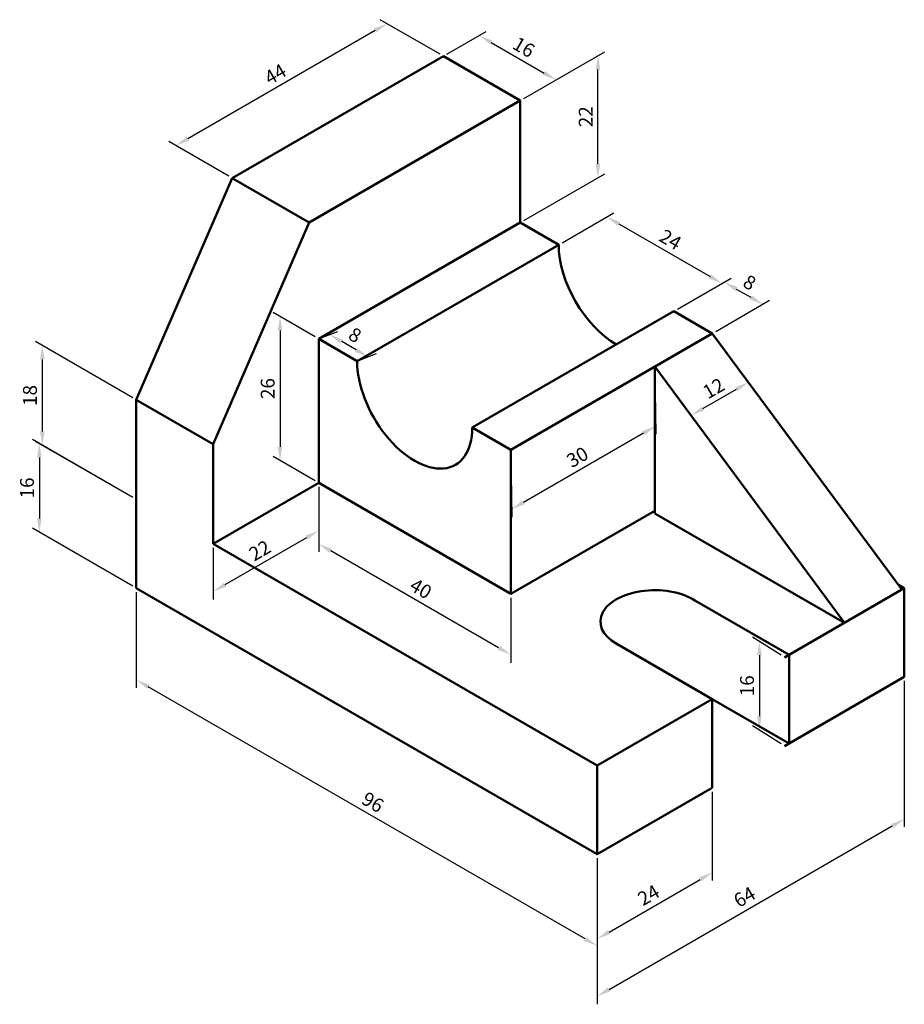
# Model space of a CAD drawing. Units: millimetres. Extents: x 27507 to 27667, y 10668 to 10845.
import ezdxf

# ---------------------------------------------------------------- set-up
doc = ezdxf.new("R2010")
doc.units = ezdxf.units.MM
doc.layers.add('M-DIMS', color=2, linetype='Continuous', lineweight=25)
doc.layers.add('M-OUTL', color=7, linetype='Continuous', lineweight=50)
doc.styles.get("Standard").update_dxf_attribs({"font": 'arial.ttf'})
doc.dimstyles.new('ISO-25', dxfattribs={"dimtxt": 2.5, "dimasz": 2.5, "dimexe": 1.25, "dimexo": 0.625, "dimtad": 1, "dimtxsty": 'Standard', "dimcen": 2.5, "dimadec": 0, "dimazin": 0, "dimtfac": 1, "dimtmove": 0, "dimatfit": 3, "dimfxl": 1, "dimarcsym": 0})

# ---------------------------------------------------------------- blocks, each defined once
blk = doc.blocks.new('*D1')
at = {"layer": 'Defpoints', "color": 0, "transparency": 16777216}
for p in [(27528.09, 10742.67), (27528.09, 10726.14), (27611.23, 10694.67)]:
    blk.add_point(p, dxfattribs=at)
at = {"layer": 'M-DIMS', "color": 0, "lineweight": -2, "transparency": 16777216}
for p, q in [((27528.09, 10741.95), (27528.09, 10724.69)), ((27609.06, 10679.39), (27530.26, 10724.89)), ((27611.23, 10693.95), (27611.23, 10676.69))]:
    blk.add_line(p, q, dxfattribs=at)
at = {"layer": 'M-DIMS', "color": 0, "transparency": 16777216}
for points in [[(27530.46, 10725.25), (27530.05, 10724.53), (27528.09, 10726.14)], [(27609.27, 10679.75), (27608.86, 10679.03), (27611.23, 10678.14)]]:
    blk.add_solid(points, dxfattribs=at)
at = {"layer": 'M-DIMS', "color": 0, "transparency": 16777216, "insert": (27570.61, 10703.78), "char_height": 2.5, "attachment_point": 5, "rotation": 330}
blk.add_mtext('96', dxfattribs=at)
blk = doc.blocks.new('*D2')
at = {"layer": 'Defpoints', "color": 0, "transparency": 16777216}
for p in [(27632.01, 10706.67), (27611.23, 10694.67), (27632.01, 10691.38)]:
    blk.add_point(p, dxfattribs=at)
at = {"layer": 'M-DIMS', "color": 0, "lineweight": -2, "transparency": 16777216}
for p, q in [((27632.01, 10705.95), (27632.01, 10689.94)), ((27611.23, 10693.95), (27611.23, 10677.94)), ((27613.39, 10680.63), (27629.85, 10690.13))]:
    blk.add_line(p, q, dxfattribs=at)
at = {"layer": 'M-DIMS', "color": 0, "transparency": 16777216}
for points in [[(27629.64, 10690.49), (27630.06, 10689.77), (27632.01, 10691.38)], [(27613.19, 10680.99), (27613.6, 10680.27), (27611.23, 10679.38)]]:
    blk.add_solid(points, dxfattribs=at)
at = {"layer": 'M-DIMS', "color": 0, "transparency": 16777216, "insert": (27620.68, 10687.01), "char_height": 2.5, "attachment_point": 5, "rotation": 30}
blk.add_mtext('24', dxfattribs=at)
blk = doc.blocks.new('*D3')
at = {"layer": 'Defpoints', "color": 0, "transparency": 16777216}
for p in [(27645.04, 10730.19), (27640.5, 10717.07), (27645.04, 10714.19)]:
    blk.add_point(p, dxfattribs=at)
at = {"layer": 'M-DIMS', "color": 0, "lineweight": -2, "transparency": 16777216}
for p, q in [((27644.41, 10730.58), (27639.25, 10733.86)), ((27640.5, 10730.57), (27640.5, 10719.57)), ((27644.41, 10714.58), (27639.25, 10717.86))]:
    blk.add_line(p, q, dxfattribs=at)
at = {"layer": 'M-DIMS', "color": 0, "transparency": 16777216}
for points in [[(27640.09, 10730.57), (27640.92, 10730.57), (27640.5, 10733.07)], [(27640.09, 10719.57), (27640.92, 10719.57), (27640.5, 10717.07)]]:
    blk.add_solid(points, dxfattribs=at)
at = {"layer": 'M-DIMS', "color": 0, "transparency": 16777216, "insert": (27638.6, 10725.07), "char_height": 2.5, "attachment_point": 5, "rotation": 90}
blk.add_mtext('16', dxfattribs=at)
blk = doc.blocks.new('*D4')
at = {"layer": 'Defpoints', "color": 0, "transparency": 16777216}
for p in [(27666.65, 10726.67), (27666.65, 10701.03), (27611.23, 10694.67)]:
    blk.add_point(p, dxfattribs=at)
at = {"layer": 'M-DIMS', "color": 0, "lineweight": -2, "transparency": 16777216}
for p, q in [((27666.65, 10725.95), (27666.65, 10699.59)), ((27613.39, 10670.28), (27664.49, 10699.78)), ((27611.23, 10693.95), (27611.23, 10667.59))]:
    blk.add_line(p, q, dxfattribs=at)
at = {"layer": 'M-DIMS', "color": 0, "transparency": 16777216}
for points in [[(27664.28, 10700.14), (27664.7, 10699.42), (27666.65, 10701.03)], [(27613.19, 10670.64), (27613.6, 10669.92), (27611.23, 10669.03)]]:
    blk.add_solid(points, dxfattribs=at)
at = {"layer": 'M-DIMS', "color": 0, "transparency": 16777216, "insert": (27637.99, 10686.68), "char_height": 2.5, "attachment_point": 5, "rotation": 30}
blk.add_mtext('64', dxfattribs=at)
blk = doc.blocks.new('*D5')
at = {"layer": 'Defpoints', "color": 0, "transparency": 16777216}
for p in [(27632.01, 10788.67), (27621.62, 10782.67), (27638.55, 10779.84)]:
    blk.add_point(p, dxfattribs=at)
at = {"layer": 'M-DIMS', "color": 0, "lineweight": -2, "transparency": 16777216}
for p, q in [((27632.39, 10788.16), (27639.29, 10778.83)), ((27621.99, 10782.16), (27628.9, 10772.83)), ((27630.32, 10775.09), (27636.38, 10778.59))]:
    blk.add_line(p, q, dxfattribs=at)
at = {"layer": 'M-DIMS', "color": 0, "transparency": 16777216}
for points in [[(27636.17, 10778.95), (27636.59, 10778.23), (27638.55, 10779.84)], [(27630.11, 10775.45), (27630.53, 10774.73), (27628.15, 10773.84)]]:
    blk.add_solid(points, dxfattribs=at)
at = {"layer": 'M-DIMS', "color": 0, "transparency": 16777216, "insert": (27632.41, 10778.47), "char_height": 2.5, "attachment_point": 5, "rotation": 30}
blk.add_mtext('12', dxfattribs=at)
blk = doc.blocks.new('*D6')
at = {"layer": 'Defpoints', "color": 0, "transparency": 16777216}
for p in [(27641.11, 10793.92), (27625.08, 10792.67), (27632.01, 10788.67)]:
    blk.add_point(p, dxfattribs=at)
at = {"layer": 'M-DIMS', "color": 0, "lineweight": -2, "transparency": 16777216}
for p, q in [((27625.71, 10793.03), (27635.43, 10798.64)), ((27636.34, 10796.67), (27638.94, 10795.17)), ((27632.64, 10789.03), (27642.36, 10794.64))]:
    blk.add_line(p, q, dxfattribs=at)
at = {"layer": 'M-DIMS', "color": 0, "transparency": 16777216}
for points in [[(27636.55, 10797.03), (27636.14, 10796.31), (27634.18, 10797.92)], [(27639.15, 10795.53), (27638.73, 10794.81), (27641.11, 10793.92)]]:
    blk.add_solid(points, dxfattribs=at)
at = {"layer": 'M-DIMS', "color": 0, "transparency": 16777216, "insert": (27638.59, 10797.57), "char_height": 2.5, "attachment_point": 5, "rotation": 330}
blk.add_mtext('8', dxfattribs=at)
blk = doc.blocks.new('*D7')
at = {"layer": 'Defpoints', "color": 0, "transparency": 16777216}
for p in [(27604.3, 10804.67), (27633.76, 10797.68), (27625.08, 10792.67)]:
    blk.add_point(p, dxfattribs=at)
at = {"layer": 'M-DIMS', "color": 0, "lineweight": -2, "transparency": 16777216}
for p, q in [((27604.93, 10805.03), (27614.23, 10810.4)), ((27615.14, 10808.43), (27631.6, 10798.93)), ((27625.71, 10793.03), (27635.01, 10798.4))]:
    blk.add_line(p, q, dxfattribs=at)
at = {"layer": 'M-DIMS', "color": 0, "transparency": 16777216}
for points in [[(27615.35, 10808.79), (27614.93, 10808.07), (27612.98, 10809.68)], [(27631.81, 10799.29), (27631.39, 10798.57), (27633.76, 10797.68)]]:
    blk.add_solid(points, dxfattribs=at)
at = {"layer": 'M-DIMS', "color": 0, "transparency": 16777216, "insert": (27624.31, 10805.31), "char_height": 2.5, "attachment_point": 5, "rotation": 330}
blk.add_mtext('24', dxfattribs=at)
blk = doc.blocks.new('*D8')
at = {"layer": 'Defpoints', "color": 0, "transparency": 16777216}
for p in [(27611.38, 10838.76), (27597.37, 10830.67), (27597.37, 10808.67)]:
    blk.add_point(p, dxfattribs=at)
at = {"layer": 'M-DIMS', "color": 0, "lineweight": -2, "transparency": 16777216}
for p, q in [((27598, 10831.03), (27612.63, 10839.48)), ((27611.38, 10819.26), (27611.38, 10836.26)), ((27598, 10809.03), (27612.63, 10817.48))]:
    blk.add_line(p, q, dxfattribs=at)
at = {"layer": 'M-DIMS', "color": 0, "transparency": 16777216}
for points in [[(27610.96, 10836.26), (27611.8, 10836.26), (27611.38, 10838.76)], [(27610.96, 10819.26), (27611.8, 10819.26), (27611.38, 10816.76)]]:
    blk.add_solid(points, dxfattribs=at)
at = {"layer": 'M-DIMS', "color": 0, "transparency": 16777216, "insert": (27609.5, 10827.76), "char_height": 2.5, "attachment_point": 5, "rotation": 90}
blk.add_mtext('22', dxfattribs=at)
blk = doc.blocks.new('*D9')
at = {"layer": 'Defpoints', "color": 0, "transparency": 16777216}
for p in [(27583.52, 10838.67), (27603.83, 10834.4), (27597.37, 10830.67)]:
    blk.add_point(p, dxfattribs=at)
at = {"layer": 'M-DIMS', "color": 0, "lineweight": -2, "transparency": 16777216}
for p, q in [((27584.14, 10839.03), (27591.22, 10843.12)), ((27592.14, 10841.15), (27601.66, 10835.65)), ((27598, 10831.03), (27605.08, 10835.12))]:
    blk.add_line(p, q, dxfattribs=at)
at = {"layer": 'M-DIMS', "color": 0, "transparency": 16777216}
for points in [[(27592.35, 10841.51), (27591.93, 10840.79), (27589.97, 10842.4)], [(27601.87, 10836.01), (27601.46, 10835.29), (27603.83, 10834.4)]]:
    blk.add_solid(points, dxfattribs=at)
at = {"layer": 'M-DIMS', "color": 0, "transparency": 16777216, "insert": (27597.85, 10840.04), "char_height": 2.5, "attachment_point": 5, "rotation": 330}
blk.add_mtext('16', dxfattribs=at)
blk = doc.blocks.new('*D10')
at = {"layer": 'Defpoints', "color": 0, "transparency": 16777216}
for p in [(27583.52, 10838.67), (27535.22, 10822.55), (27545.41, 10816.67)]:
    blk.add_point(p, dxfattribs=at)
at = {"layer": 'M-DIMS', "color": 0, "lineweight": -2, "transparency": 16777216}
for p, q in [((27582.89, 10839.03), (27572.08, 10845.27)), ((27571.16, 10843.3), (27537.39, 10823.8)), ((27544.79, 10817.03), (27533.97, 10823.27))]:
    blk.add_line(p, q, dxfattribs=at)
at = {"layer": 'M-DIMS', "color": 0, "transparency": 16777216}
for points in [[(27570.96, 10843.66), (27571.37, 10842.94), (27573.33, 10844.55)], [(27537.18, 10824.16), (27537.6, 10823.44), (27535.22, 10822.55)]]:
    blk.add_solid(points, dxfattribs=at)
at = {"layer": 'M-DIMS', "color": 0, "transparency": 16777216, "insert": (27553.34, 10835.17), "char_height": 2.5, "attachment_point": 5, "rotation": 30}
blk.add_mtext('44', dxfattribs=at)
blk = doc.blocks.new('*D11')
at = {"layer": 'Defpoints', "color": 0, "transparency": 16777216}
for p in [(27528.09, 10776.67), (27511.13, 10768.46), (27528.09, 10758.67)]:
    blk.add_point(p, dxfattribs=at)
at = {"layer": 'M-DIMS', "color": 0, "lineweight": -2, "transparency": 16777216}
for p, q in [((27527.46, 10777.03), (27509.88, 10787.18)), ((27511.13, 10783.96), (27511.13, 10770.96)), ((27527.46, 10759.03), (27509.88, 10769.18))]:
    blk.add_line(p, q, dxfattribs=at)
at = {"layer": 'M-DIMS', "color": 0, "transparency": 16777216}
for points in [[(27510.72, 10783.96), (27511.55, 10783.96), (27511.13, 10786.46)], [(27510.72, 10770.96), (27511.55, 10770.96), (27511.13, 10768.46)]]:
    blk.add_solid(points, dxfattribs=at)
at = {"layer": 'M-DIMS', "color": 0, "transparency": 16777216, "insert": (27509.23, 10777.46), "char_height": 2.5, "attachment_point": 5, "rotation": 90}
blk.add_mtext('18', dxfattribs=at)
blk = doc.blocks.new('*D12')
at = {"layer": 'Defpoints', "color": 0, "transparency": 16777216}
for p in [(27528.09, 10758.67), (27510.6, 10752.77), (27528.09, 10742.67)]:
    blk.add_point(p, dxfattribs=at)
at = {"layer": 'M-DIMS', "color": 0, "lineweight": -2, "transparency": 16777216}
for p, q in [((27527.46, 10759.03), (27509.35, 10769.49)), ((27510.6, 10766.27), (27510.6, 10755.27)), ((27527.46, 10743.03), (27509.35, 10753.49))]:
    blk.add_line(p, q, dxfattribs=at)
at = {"layer": 'M-DIMS', "color": 0, "transparency": 16777216}
for points in [[(27510.18, 10766.27), (27511.01, 10766.27), (27510.6, 10768.77)], [(27510.18, 10755.27), (27511.01, 10755.27), (27510.6, 10752.77)]]:
    blk.add_solid(points, dxfattribs=at)
at = {"layer": 'M-DIMS', "color": 0, "transparency": 16777216, "insert": (27508.7, 10760.77), "char_height": 2.5, "attachment_point": 5, "rotation": 90}
blk.add_mtext('16', dxfattribs=at)
blk = doc.blocks.new('*D13')
at = {"layer": 'Defpoints', "color": 0, "transparency": 16777216}
for p in [(27561, 10761.67), (27561, 10753.07), (27541.95, 10750.67)]:
    blk.add_point(p, dxfattribs=at)
at = {"layer": 'M-DIMS', "color": 0, "lineweight": -2, "transparency": 16777216}
for p, q in [((27561, 10760.95), (27561, 10751.63)), ((27544.11, 10743.32), (27558.83, 10751.82)), ((27541.95, 10749.95), (27541.95, 10740.63))]:
    blk.add_line(p, q, dxfattribs=at)
at = {"layer": 'M-DIMS', "color": 0, "transparency": 16777216}
for points in [[(27558.63, 10752.18), (27559.04, 10751.46), (27561, 10753.07)], [(27543.9, 10743.68), (27544.32, 10742.96), (27541.95, 10742.07)]]:
    blk.add_solid(points, dxfattribs=at)
at = {"layer": 'M-DIMS', "color": 0, "transparency": 16777216, "insert": (27550.53, 10749.2), "char_height": 2.5, "attachment_point": 5, "rotation": 30}
blk.add_mtext('22', dxfattribs=at)
blk = doc.blocks.new('*D14')
at = {"layer": 'Defpoints', "color": 0, "transparency": 16777216}
for p in [(27561, 10761.67), (27561, 10750.67), (27595.64, 10741.67)]:
    blk.add_point(p, dxfattribs=at)
at = {"layer": 'M-DIMS', "color": 0, "lineweight": -2, "transparency": 16777216}
for p, q in [((27561, 10760.95), (27561, 10749.23)), ((27593.47, 10731.92), (27563.16, 10749.42)), ((27595.64, 10740.95), (27595.64, 10729.23))]:
    blk.add_line(p, q, dxfattribs=at)
at = {"layer": 'M-DIMS', "color": 0, "transparency": 16777216}
for points in [[(27563.37, 10749.78), (27562.96, 10749.06), (27561, 10750.67)], [(27593.68, 10732.28), (27593.27, 10731.56), (27595.64, 10730.67)]]:
    blk.add_solid(points, dxfattribs=at)
at = {"layer": 'M-DIMS', "color": 0, "transparency": 16777216, "insert": (27579.27, 10742.32), "char_height": 2.5, "attachment_point": 5, "rotation": 330}
blk.add_mtext('40', dxfattribs=at)
blk = doc.blocks.new('*D15')
at = {"layer": 'Defpoints', "color": 0, "transparency": 16777216}
for p in [(27561, 10787.67), (27554.02, 10765.7), (27561, 10761.67)]:
    blk.add_point(p, dxfattribs=at)
at = {"layer": 'M-DIMS', "color": 0, "lineweight": -2, "transparency": 16777216}
for p, q in [((27560.37, 10788.03), (27552.77, 10792.42)), ((27554.02, 10789.2), (27554.02, 10768.2)), ((27560.37, 10762.03), (27552.77, 10766.42))]:
    blk.add_line(p, q, dxfattribs=at)
at = {"layer": 'M-DIMS', "color": 0, "transparency": 16777216}
for points in [[(27553.6, 10789.2), (27554.44, 10789.2), (27554.02, 10791.7)], [(27553.6, 10768.2), (27554.44, 10768.2), (27554.02, 10765.7)]]:
    blk.add_solid(points, dxfattribs=at)
at = {"layer": 'M-DIMS', "color": 0, "transparency": 16777216, "insert": (27552.12, 10778.7), "char_height": 2.5, "attachment_point": 5, "rotation": 90}
blk.add_mtext('26', dxfattribs=at)
blk = doc.blocks.new('*D16')
at = {"layer": 'Defpoints', "color": 0, "transparency": 16777216}
for p in [(27561, 10787.67), (27562.98, 10788.43), (27567.93, 10783.67)]:
    blk.add_point(p, dxfattribs=at)
at = {"layer": 'M-DIMS', "color": 0, "lineweight": -2, "transparency": 16777216}
for p, q in [((27561.75, 10787.96), (27564.48, 10789.01)), ((27567.75, 10785.68), (27565.15, 10787.18)), ((27568.68, 10783.96), (27571.41, 10785.01))]:
    blk.add_line(p, q, dxfattribs=at)
at = {"layer": 'M-DIMS', "color": 0, "transparency": 16777216}
for points in [[(27565.36, 10787.54), (27564.94, 10786.82), (27562.98, 10788.43)], [(27567.95, 10786.04), (27567.54, 10785.32), (27569.91, 10784.43)]]:
    blk.add_solid(points, dxfattribs=at)
at = {"layer": 'M-DIMS', "color": 0, "transparency": 16777216, "insert": (27567.4, 10788.08), "char_height": 2.5, "attachment_point": 5, "rotation": 330}
blk.add_mtext('8', dxfattribs=at)
blk = doc.blocks.new('*D17')
at = {"layer": 'Defpoints', "color": 0, "transparency": 16777216}
for p in [(27621.62, 10782.67), (27595.64, 10767.67), (27595.8, 10756.91)]:
    blk.add_point(p, dxfattribs=at)
at = {"layer": 'M-DIMS', "color": 0, "lineweight": -2, "transparency": 16777216}
for p, q in [((27621.63, 10781.95), (27621.8, 10770.48)), ((27619.61, 10770.66), (27597.96, 10758.16)), ((27595.65, 10766.95), (27595.82, 10755.48))]:
    blk.add_line(p, q, dxfattribs=at)
at = {"layer": 'M-DIMS', "color": 0, "transparency": 16777216}
for points in [[(27619.4, 10771.03), (27619.82, 10770.3), (27621.78, 10771.91)], [(27597.75, 10758.53), (27598.17, 10757.8), (27595.8, 10756.91)]]:
    blk.add_solid(points, dxfattribs=at)
at = {"layer": 'M-DIMS', "color": 0, "transparency": 16777216, "insert": (27607.84, 10766.06), "char_height": 2.5, "attachment_point": 5, "rotation": 30}
blk.add_mtext('30', dxfattribs=at)

msp = doc.modelspace()

# ---------------------------------------------------------------- linework, layer by layer
at = {"layer": 'M-OUTL'}
for p, q in [((27545.41, 10816.668), (27583.516, 10838.668)), ((27583.516, 10838.668), (27597.372, 10830.668)), ((27597.372, 10830.668), (27559.267, 10808.668)), ((27597.372, 10830.668), (27597.372, 10808.668)), ((27545.41, 10816.668), (27528.09, 10776.668)), ((27559.267, 10808.668), (27545.41, 10816.668)), ((27559.267, 10808.668), (27541.946, 10768.668)), ((27560.999, 10787.668), (27597.372, 10808.668)), ((27597.372, 10808.668), (27604.3, 10804.668)), ((27604.3, 10804.668), (27597.372, 10808.668)), ((27567.927, 10783.668), (27604.3, 10804.668)), ((27625.085, 10792.668), (27588.712, 10771.668)), ((27632.013, 10788.668), (27625.085, 10792.668)), ((27560.999, 10787.668), (27567.927, 10783.668)), ((27560.999, 10787.668), (27560.999, 10761.668)), ((27595.64, 10767.668), (27632.013, 10788.668)), ((27632.013, 10788.668), (27621.621, 10782.668)), ((27632.013, 10788.668), (27666.237, 10742.428)), ((27621.621, 10782.668), (27621.621, 10756.187)), ((27621.621, 10782.668), (27655.845, 10736.428)), ((27528.09, 10742.668), (27528.09, 10776.668)), ((27528.09, 10776.668), (27541.946, 10768.668)), ((27588.712, 10771.668), (27595.64, 10767.668)), ((27541.946, 10768.668), (27541.946, 10750.668)), ((27595.64, 10767.668), (27595.64, 10741.668)), ((27541.946, 10750.668), (27560.999, 10761.668)), ((27560.999, 10761.668), (27595.64, 10741.668)), ((27528.09, 10758.668), (27528.09, 10742.668)), ((27595.64, 10741.668), (27621.621, 10756.668)), ((27621.621, 10756.187), (27655.845, 10736.428)), ((27611.228, 10710.668), (27541.946, 10750.668)), ((27665.614, 10743.269), (27666.654, 10742.668)), ((27611.228, 10694.668), (27528.09, 10742.668)), ((27666.654, 10742.668), (27645.035, 10730.187)), ((27666.654, 10742.668), (27666.654, 10726.668)), ((27645.869, 10730.668), (27628.549, 10740.668)), ((27632.013, 10722.668), (27614.693, 10732.668)), ((27645.869, 10714.668), (27645.869, 10730.668)), ((27666.654, 10726.668), (27645.035, 10714.187)), ((27611.228, 10710.668), (27632.013, 10722.668)), ((27632.013, 10722.668), (27611.228, 10710.668)), ((27632.013, 10722.668), (27632.013, 10706.668)), ((27645.869, 10714.668), (27632.013, 10722.668)), ((27611.228, 10710.668), (27611.228, 10694.668)), ((27632.013, 10706.668), (27611.228, 10694.668))]:
    msp.add_line(p, q, dxfattribs=at)
for centre, major_axis, start_param, end_param in [((27614.693, 10798.668), (7.348, -12.728), 3.9269908, 5.4977871), ((27578.319, 10777.668), (7.348, -12.728), 3.9269908, 7.0685835), ((27621.621, 10736.668), (-9.798, 0), 3.8107672, 7.0685835)]:
    msp.add_ellipse(centre, major_axis=major_axis, ratio=0.5773503, start_param=start_param, end_param=end_param, dxfattribs=at)

# ---------------------------------------------------------------- dimensions: what is measured, and where the dimension line sits
at = {"layer": 'M-DIMS'}
for p1, p2, distance, picture, middle in [((27583.516, 10838.668), (27545.41, 10816.668), -10.187, '*D10', (27553.339, 10835.174)), ((27583.516, 10838.668), (27597.372, 10830.668), 6.456, '*D9', (27597.851, 10840.043)), ((27597.372, 10808.668), (27597.372, 10830.668), -14.007, '*D8', (27609.499, 10827.756)), ((27604.3, 10804.668), (27625.085, 10792.668), 8.678, '*D7', (27624.31, 10805.307)), ((27625.085, 10792.668), (27632.013, 10788.668), 9.094, '*D6', (27638.594, 10797.566)), ((27560.999, 10787.668), (27560.999, 10761.668), -6.977, '*D15', (27552.12, 10778.697)), ((27567.927, 10783.668), (27560.999, 10787.668), -1.653, '*D16', (27567.398, 10788.078)), ((27621.621, 10782.668), (27632.013, 10788.668), -10.909, '*D5', (27632.409, 10778.471)), ((27528.09, 10776.668), (27528.09, 10758.668), -16.957, '*D11', (27509.232, 10777.459)), ((27621.621, 10782.668), (27595.64, 10767.668), 9.391, '*D17', (27607.835, 10766.062)), ((27528.09, 10758.668), (27528.09, 10742.668), -17.493, '*D12', (27508.696, 10760.768)), ((27541.946, 10750.668), (27560.999, 10761.668), -7.443, '*D13', (27550.533, 10749.202)), ((27595.64, 10741.668), (27560.999, 10761.668), 9.526, '*D14', (27579.27, 10742.315)), ((27611.228, 10694.668), (27528.09, 10742.668), 14.317, '*D1', (27570.61, 10703.783)), ((27645.035, 10730.187), (27645.035, 10714.187), -4.533, '*D3', (27638.601, 10725.066)), ((27611.228, 10694.668), (27666.654, 10726.668), -22.205, '*D4', (27637.991, 10686.675)), ((27611.228, 10694.668), (27632.013, 10706.668), -13.241, '*D2', (27620.681, 10687.007))]:
    dim = msp.add_aligned_dim(p1=p1, p2=p2, distance=distance, dimstyle='ISO-25', override={"dimclrd": 0, "dimclre": 0, "dimclrt": 0}, dxfattribs=at)
    dim.commit()
    dim.dimension.update_dxf_attribs({"geometry": picture, "text_midpoint": middle})

doc.saveas('drawing.dxf')
